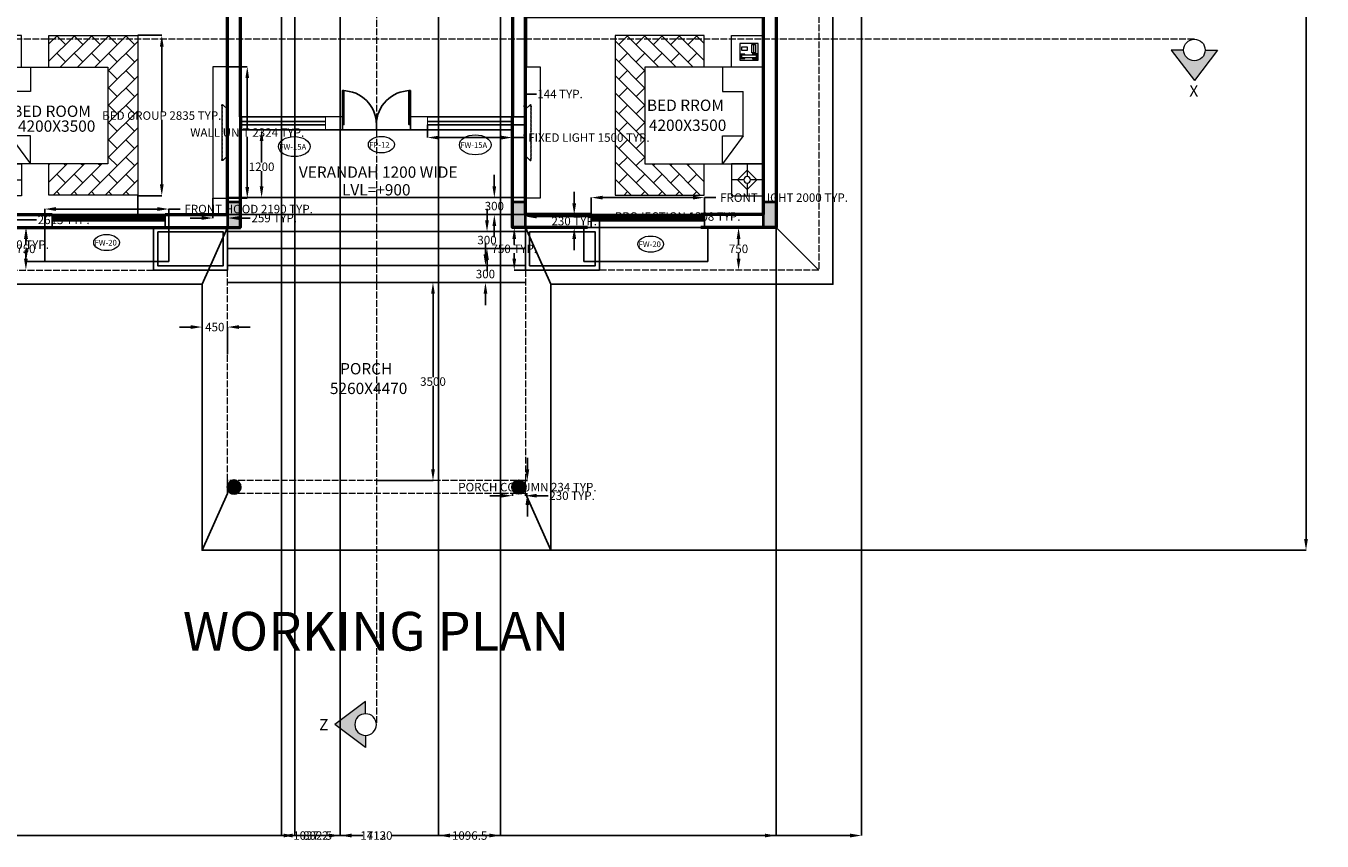
# Model space of a CAD drawing. Units: inches. Extents: x 22626 to 57351, y 2118 to 36234.
# Tile 3 of 10: x 34432 to 57323, y 2118 to 16521. Entities that reach past the tile are written whole.
import ezdxf

# ---------------------------------------------------------------- set-up
doc = ezdxf.new("R2010")
doc.units = ezdxf.units.IN
doc.header["$MEASUREMENT"] = 0
doc.linetypes.add('ACAD_ISO02W100', pattern=[15, 12, -3])
for name, color, linetype, lineweight in [('A-ANNO-DIMS', 130, 'Continuous', 18), ('A-ANNO-IDEN', 130, 'Continuous', 15), ('A-ANNO-SYMB', 130, 'Continuous', 18), ('A-ANNO-TITL', 130, 'Continuous', 35), ('A-AREA-IDEN', 130, 'Continuous', 18), ('A-COLS', 7, 'Continuous', 40), ('A-ROOF', 80, 'Continuous', 25), ('A-ROOF-OVHD', 80, 'ACAD_ISO02W100', 18), ('A-WALL', 80, 'Continuous', 50), ('DOORS', 32, 'Continuous', 25), ('FURNITURE', 30, 'Continuous', 18), ('STAIRS', 82, 'Continuous', 25), ('WINDOWS', 212, 'Continuous', 25)]:
    doc.layers.add(name, color=color, linetype=linetype, lineweight=lineweight)
doc.layers.add('A-SECT', color=2, linetype='ACAD_ISO02W100', lineweight=18, true_color=0xf1eb1f)
doc.styles.get("Standard").update_dxf_attribs({"font": 'arial.ttf'})
doc.dimstyles.get("Standard").update_dxf_attribs({"dimtxt": 150, "dimasz": 200, "dimexe": 0.18, "dimexo": 0.0625, "dimgap": 0.09, "dimtad": 0, "dimtih": 1, "dimtoh": 1, "dimdec": 0, "dimzin": 0, "dimdsep": 46, "dimtxsty": 'Standard', "dimcen": 0.09, "dimadec": 0, "dimazin": 0, "dimtfac": 1, "dimtdec": 0, "dimtofl": 0, "dimtmove": 0, "dimatfit": 3, "dimfxl": 1, "dimtolj": 1, "dimtzin": 0, "dimarcsym": 0})

# ---------------------------------------------------------------- blocks, each defined once
blk = doc.blocks.new('*D1')
at = {"layer": 'A-ANNO-DIMS', "color": 0, "lineweight": -2, "transparency": 16777216}
for p, q in [((40622, 11987), (41621, 11987)), ((41621, 11787), (41621, 10314)), ((41621, 8687), (41621, 10160)), ((40622, 8487), (41621, 8487))]:
    blk.add_line(p, q, dxfattribs=at)
at = {"layer": 'A-ANNO-DIMS', "color": 0, "transparency": 16777216}
for points in [[(41587, 11787), (41654, 11787), (41621, 11987)], [(41587, 8687), (41654, 8687), (41621, 8487)]]:
    blk.add_solid(points, dxfattribs=at)
at = {"layer": 'Defpoints', "color": 0, "transparency": 16777216}
for p in [(40622, 11987), (40622, 8487), (41621, 8487)]:
    blk.add_point(p, dxfattribs=at)
at = {"layer": 'A-ANNO-DIMS', "color": 0, "transparency": 16777216, "insert": (41621, 10237), "char_height": 150, "attachment_point": 5}
blk.add_mtext('\\A1;3500', dxfattribs=at)
blk = doc.blocks.new('*D2')
at = {"layer": 'A-ANNO-DIMS', "color": 0, "lineweight": -2, "transparency": 16777216}
for p, q in [((37342, 11200), (37142, 11200)), ((37542, 10722), (37542, 11200)), ((37992, 10722), (37992, 11200)), ((38192, 11200), (38392, 11200))]:
    blk.add_line(p, q, dxfattribs=at)
at = {"layer": 'A-ANNO-DIMS', "color": 0, "transparency": 16777216}
for points in [[(37342, 11233), (37342, 11167), (37542, 11200)], [(38192, 11233), (38192, 11167), (37992, 11200)]]:
    blk.add_solid(points, dxfattribs=at)
at = {"layer": 'Defpoints', "color": 0, "transparency": 16777216}
for p in [(37542, 11200), (37542, 10722), (37992, 10722)]:
    blk.add_point(p, dxfattribs=at)
at = {"layer": 'A-ANNO-DIMS', "color": 0, "transparency": 16777216, "insert": (37767, 11200), "char_height": 150, "attachment_point": 5}
blk.add_mtext('\\A1;450', dxfattribs=at)
blk = doc.blocks.new('*D3')
at = {"layer": 'A-ANNO-DIMS', "color": 0, "lineweight": -2, "transparency": 16777216}
for p, q in [((42547, 12487), (42547, 12687)), ((43252, 12287), (42547, 12287)), ((43252, 11987), (42547, 11987)), ((42547, 11787), (42547, 11587))]:
    blk.add_line(p, q, dxfattribs=at)
at = {"layer": 'A-ANNO-DIMS', "color": 0, "transparency": 16777216}
for points in [[(42514, 12487), (42581, 12487), (42547, 12287)], [(42514, 11787), (42581, 11787), (42547, 11987)]]:
    blk.add_solid(points, dxfattribs=at)
at = {"layer": 'Defpoints', "color": 0, "transparency": 16777216}
for p in [(42547, 12287), (43252, 12287), (43252, 11987)]:
    blk.add_point(p, dxfattribs=at)
at = {"layer": 'A-ANNO-DIMS', "color": 0, "transparency": 16777216, "insert": (42547, 12137), "char_height": 150, "attachment_point": 5}
blk.add_mtext('\\A1;300', dxfattribs=at)
blk = doc.blocks.new('*D4')
at = {"layer": 'A-ANNO-DIMS', "color": 0, "lineweight": -2, "transparency": 16777216}
for p, q in [((42704, 13687), (42704, 13887)), ((43252, 13487), (42704, 13487)), ((43252, 13187), (42704, 13187)), ((42704, 12987), (42704, 12787))]:
    blk.add_line(p, q, dxfattribs=at)
at = {"layer": 'A-ANNO-DIMS', "color": 0, "transparency": 16777216}
for points in [[(42671, 13687), (42737, 13687), (42704, 13487)], [(42671, 12987), (42737, 12987), (42704, 13187)]]:
    blk.add_solid(points, dxfattribs=at)
at = {"layer": 'Defpoints', "color": 0, "transparency": 16777216}
for p in [(43252, 13487), (42704, 13187), (43252, 13187)]:
    blk.add_point(p, dxfattribs=at)
at = {"layer": 'A-ANNO-DIMS', "color": 0, "transparency": 16777216, "insert": (42704, 13337), "char_height": 150, "attachment_point": 5}
blk.add_mtext('\\A1;300', dxfattribs=at)
blk = doc.blocks.new('*D5')
at = {"layer": 'A-ANNO-DIMS', "color": 0, "lineweight": -2, "transparency": 16777216}
for p, q in [((42575, 13087), (42575, 13287)), ((43252, 12887), (42574, 12887)), ((43252, 12587), (42574, 12587)), ((42575, 12387), (42575, 12187))]:
    blk.add_line(p, q, dxfattribs=at)
at = {"layer": 'A-ANNO-DIMS', "color": 0, "transparency": 16777216}
for points in [[(42541, 13087), (42608, 13087), (42575, 12887)], [(42541, 12387), (42608, 12387), (42575, 12587)]]:
    blk.add_solid(points, dxfattribs=at)
at = {"layer": 'Defpoints', "color": 0, "transparency": 16777216}
for p in [(43252, 12887), (42575, 12587), (43252, 12587)]:
    blk.add_point(p, dxfattribs=at)
at = {"layer": 'A-ANNO-DIMS', "color": 0, "transparency": 16777216, "insert": (42575, 12737), "char_height": 150, "attachment_point": 5}
blk.add_mtext('\\A1;300', dxfattribs=at)
blk = doc.blocks.new('Phone - Desk')
for p, q in [((-4.5, -5), (-4.5, 5)), ((-4.5, 5), (4.5, 5)), ((-4, 4.5), (-4, 2)), ((-4, 2), (-3.25, 2)), ((-3.75, 4.5), (-3.75, 2.25)), ((-1.25, 4.5), (-3.75, 4.5)), ((-3.75, 2.25), (-3.25, 2.25)), ((-3.25, 4), (-3.25, -4)), ((-3.25, 4), (-1.75, 4)), ((-1.75, -4), (-1.75, 4)), ((-1.75, 2.25), (-1.25, 2.25)), ((-1.75, 2), (-1, 2)), ((-1.25, 2.25), (-1.25, 4.5)), ((-1, 2), (-1, 4.5)), ((4, 3.5), (-0.5, 3.5)), ((-0.5, 3.5), (-0.5, 1.5)), ((-0.5, 2.5), (4, 2.5)), ((-0.5, 1.5), (4, 1.5)), ((4, 1.5), (4, 3.5)), ((4.5, 5), (4.5, -5)), ((4.5, -5), (-4.5, -5)), ((-3.75, -2.25), (-3.25, -2.25)), ((-3.75, -4.5), (-3.75, -2.25)), ((-1.25, -4.5), (-3.75, -4.5)), ((-3.25, -4), (-1.75, -4)), ((-1.75, -2.25), (-1.25, -2.25)), ((-1.25, -2.25), (-1.25, -4.5)), ((2.75, -1), (0.75, -1)), ((0.75, -1), (0.75, -4)), ((0.75, -4), (2.75, -4)), ((2.75, -4), (2.75, -1))]:
    blk.add_line(p, q)
blk = doc.blocks.new('BED')
h = blk.add_hatch()
h.set_pattern_fill('AR-B816', color=256, scale=27, angle=45)
h.paths.add_polyline_path([(36405, 26901), (36405, 25191), (35361, 25191), (35361, 24640), (36931, 24640), (36931, 25191), (36931, 27463), (36405, 27463), (35361, 27463), (35361, 26901)])
for p, q in [((35361, 26901), (35361, 27463)), ((35361, 27463), (36405, 27463)), ((36405, 27463), (36931, 27463)), ((36931, 27463), (36931, 25191)), ((35035, 26901), (35035, 26469)), ((34673, 25686), (34673, 26469)), ((35035, 26469), (34673, 26469)), ((35035, 25686), (34673, 25686)), ((34673, 25686), (35035, 25191)), ((35035, 25191), (35035, 25686)), ((34599, 25191), (34599, 24968)), ((35361, 24640), (35361, 25191)), ((36931, 25191), (36931, 24640)), ((34429, 24909), (34599, 25080)), ((34599, 25080), (34769, 24909)), ((34317, 24909), (34540, 24909)), ((34599, 24739), (34429, 24909)), ((34769, 24909), (34599, 24739)), ((34599, 24850), (34599, 24628)), ((34658, 24909), (34880, 24909)), ((36931, 24640), (35361, 24640))]:
    blk.add_line(p, q)
for points in [[(34317, 26901), (34880, 26901), (34880, 27463), (34317, 27463)], [(34317, 26901), (36405, 26901), (36405, 25191), (34317, 25191)], [(34317, 25191), (34880, 25191), (34880, 24628), (34317, 24628)]]:
    blk.add_lwpolyline(points, close=True)
blk.add_circle((34599, 24909), 59)
at = {"xscale": 32.52267765020765, "yscale": 32.52267765020765, "zscale": 32.52267765020765, "rotation": 90}
blk.add_blockref('Phone - Desk', (34567, 27173), dxfattribs=at)
blk = doc.blocks.new('*U7')
for p, q in [((0, 0), (0, -6)), ((40, 0), (40, -6))]:
    blk.add_line(p, q)
blk.add_lwpolyline([(0, 0), (0, 40), (1.75, 40), (1.75, 0)], close=True)
blk.add_arc((0, 0), 40, 0, 90)
blk = doc.blocks.new('*D16')
at = {"layer": 'A-ANNO-DIMS', "color": 0, "lineweight": -2, "transparency": 16777216}
for p, q in [((47017, 12957), (47018, 12957)), ((47017, 12757), (47017, 12659)), ((47017, 12407), (47017, 12505)), ((47017, 12207), (47018, 12207))]:
    blk.add_line(p, q, dxfattribs=at)
at = {"layer": 'A-ANNO-DIMS', "color": 0, "transparency": 16777216}
for points in [[(46984, 12757), (47051, 12757), (47017, 12957)], [(46984, 12407), (47051, 12407), (47017, 12207)]]:
    blk.add_solid(points, dxfattribs=at)
at = {"layer": 'Defpoints', "color": 0, "transparency": 16777216}
for p in [(47017, 12957), (47017, 12207), (47017, 12207)]:
    blk.add_point(p, dxfattribs=at)
at = {"layer": 'A-ANNO-DIMS', "color": 0, "transparency": 16777216, "insert": (47017, 12582), "char_height": 150, "attachment_point": 5}
blk.add_mtext('\\A1;750', dxfattribs=at)
blk = doc.blocks.new('*D17')
at = {"layer": 'A-ANNO-DIMS', "color": 0, "lineweight": -2, "transparency": 16777216}
for p, q in [((38594, 14687), (38594, 14687)), ((38594, 14487), (38594, 14108)), ((38594, 13687), (38594, 13955)), ((38594, 13487), (38594, 13487))]:
    blk.add_line(p, q, dxfattribs=at)
at = {"layer": 'A-ANNO-DIMS', "color": 0, "transparency": 16777216}
for points in [[(38561, 14487), (38627, 14487), (38594, 14687)], [(38561, 13687), (38627, 13687), (38594, 13487)]]:
    blk.add_solid(points, dxfattribs=at)
at = {"layer": 'Defpoints', "color": 0, "transparency": 16777216}
for p in [(38594, 14687), (38594, 14687), (38594, 13487)]:
    blk.add_point(p, dxfattribs=at)
at = {"layer": 'A-ANNO-DIMS', "color": 0, "transparency": 16777216, "insert": (38594, 14032), "char_height": 150, "attachment_point": 5}
blk.add_mtext('\\A1;1200', dxfattribs=at)
blk = doc.blocks.new('*D19')
at = {"layer": 'A-ANNO-DIMS', "color": 0, "lineweight": -2, "transparency": 16777216}
for p, q in [((34431, 12957), (34431, 12957)), ((34431, 12757), (34431, 12659)), ((34431, 12407), (34431, 12505)), ((34431, 12207), (34431, 12207))]:
    blk.add_line(p, q, dxfattribs=at)
at = {"layer": 'A-ANNO-DIMS', "color": 0, "transparency": 16777216}
for points in [[(34398, 12757), (34464, 12757), (34431, 12957)], [(34398, 12407), (34464, 12407), (34431, 12207)]]:
    blk.add_solid(points, dxfattribs=at)
at = {"layer": 'Defpoints', "color": 0, "transparency": 16777216}
for p in [(34431, 12957), (34431, 12207), (34431, 12207)]:
    blk.add_point(p, dxfattribs=at)
at = {"layer": 'A-ANNO-DIMS', "color": 0, "transparency": 16777216, "insert": (34431, 12582), "char_height": 150, "attachment_point": 5}
blk.add_mtext('\\A1;750', dxfattribs=at)
blk = doc.blocks.new('BEDROOM-WALL-UNIT-SMALL')
for p, q in [((259, 1576), (175, 1654)), ((259, 1576), (259, 748)), ((259, 748), (175, 670))]:
    blk.add_line(p, q)
blk.add_lwpolyline([(259, 2324), (0, 2324), (0, 0), (259, 0)], close=True)
for centre in [(168, 1645), (168, 679)]:
    blk.add_circle(centre, 11.7)
for centre, radius, start, end in [((170, 1620), 14.3, 99.4783, 260.5217), ((168, 1594), 11.7, 90, 270), ((168, 1570), 11.7, 90, 270), ((168, 1547), 11.7, 90, 270), ((168, 1523), 11.7, 90, 270), ((168, 1500), 11.7, 90, 270), ((168, 1476), 11.7, 90, 270), ((168, 1453), 11.7, 90, 270), ((168, 1430), 11.7, 90, 270), ((168, 1406), 11.7, 90, 270), ((168, 1383), 11.7, 90, 270), ((168, 1359), 11.7, 90, 270), ((168, 1336), 11.7, 90, 270), ((168, 1312), 11.7, 90, 270), ((168, 1289), 11.7, 90, 270), ((168, 1265), 11.7, 90, 270), ((168, 1242), 11.7, 90, 270), ((168, 1218), 11.7, 90, 270), ((168, 1195), 11.7, 90, 270), ((168, 1172), 11.7, 90, 270), ((168, 1148), 11.7, 90, 270), ((168, 1125), 11.7, 90, 270), ((168, 1101), 11.7, 90, 270), ((168, 1078), 11.7, 90, 270), ((168, 1054), 11.7, 90, 270), ((168, 1031), 11.7, 90, 270), ((168, 1007), 11.7, 90, 270), ((168, 984), 11.7, 90, 270), ((168, 960), 11.7, 90, 270), ((168, 937), 11.7, 90, 270), ((168, 914), 11.7, 90, 270), ((168, 890), 11.7, 90, 270), ((168, 867), 11.7, 90, 270), ((168, 843), 11.7, 90, 270), ((168, 820), 11.7, 90, 270), ((168, 796), 11.7, 90, 270), ((168, 773), 11.7, 90, 270), ((168, 749), 11.7, 90, 270), ((168, 726), 11.7, 90, 270), ((168, 702), 11.7, 90, 270)]:
    blk.add_arc(centre, radius, start, end)
blk = doc.blocks.new('WIN-FIXED-2000-FRONT')
for p, q in [((0, 207), (2000, 207)), ((0, 177), (2000, 177)), ((0, 147), (2000, 147)), ((0, 117), (2000, 117))]:
    blk.add_line(p, q)
blk.add_lwpolyline([(0, 230), (2000, 230), (2000, 0), (0, 0), (0, 230)])
blk = doc.blocks.new('COL-RECTANGULAR')
h = blk.add_hatch(color=256)
h.dxf.hatch_style = 1
h.paths.add_polyline_path([(0, 0), (450, 0), (450, 230), (0, 230)])
blk.add_lwpolyline([(0, 0), (0, 230), (450, 230), (450, 0)], close=True)
blk = doc.blocks.new('COL-ROUND')
h = blk.add_hatch(color=256)
h.dxf.hatch_style = 1
h.paths.add_polyline_path([(0, 115, 0.970679), (230, 108), (230, 122, 0.970679)])
blk.add_circle((115, 115), 115)
blk = doc.blocks.new('SECTION-HEAD')
h = blk.add_hatch(color=256)
h.dxf.hatch_style = 1
h.paths.add_polyline_path([(815, 541), (599, 541, -1), (216, 541), (0, 541), (407, 0)])
for p, q in [((216, 541), (0, 541)), ((0, 541), (407, 0)), ((815, 541), (407, 0)), ((599, 541), (815, 541))]:
    blk.add_line(p, q)
blk.add_circle((407, 541), 191)
blk = doc.blocks.new('WINDOW-HOOD-FRONT')
for p, q in [((0, 0), (0, 600)), ((2190, 600), (2190, 0)), ((2190, 0), (0, 0))]:
    blk.add_line(p, q)
blk = doc.blocks.new('FRONT-PROJECTION')
for points in [[(0, 750), (1308, 750), (1308, 0), (0, 0)], [(75, 675), (1233, 675), (1233, 75), (75, 75)]]:
    blk.add_lwpolyline(points, close=True)
blk = doc.blocks.new('WIN-FIXED-1500')
for p, q in [((1500, 144), (0, 144)), ((0, 58), (1500, 58)), ((0, 0), (1500, 0))]:
    blk.add_line(p, q)
blk = doc.blocks.new('*D58')
at = {"layer": 'A-ANNO-DIMS', "color": 0, "lineweight": -2, "transparency": 16777216}
for p, q in [((43288, 8689), (43288, 8889)), ((43253, 8489), (43288, 8489)), ((43253, 8255), (43288, 8255)), ((43288, 8055), (43288, 7855))]:
    blk.add_line(p, q, dxfattribs=at)
at = {"layer": 'A-ANNO-DIMS', "color": 0, "transparency": 16777216}
for points in [[(43254, 8689), (43321, 8689), (43288, 8489)], [(43254, 8055), (43321, 8055), (43288, 8255)]]:
    blk.add_solid(points, dxfattribs=at)
at = {"layer": 'Defpoints', "color": 0, "transparency": 16777216}
for p in [(43253, 8489), (43288, 8489), (43253, 8255)]:
    blk.add_point(p, dxfattribs=at)
at = {"layer": 'A-ANNO-DIMS', "color": 0, "transparency": 16777216, "insert": (43288, 8372), "char_height": 150, "attachment_point": 5}
blk.add_mtext('\\A1;PORCH COLUMN 234 TYP.', dxfattribs=at)
blk = doc.blocks.new('*D59')
at = {"layer": 'A-ANNO-DIMS', "color": 0, "lineweight": -2, "transparency": 16777216}
for p, q in [((43023, 8255), (43023, 8220)), ((43253, 8255), (43253, 8220)), ((42823, 8220), (42623, 8220)), ((43453, 8220), (43653, 8220))]:
    blk.add_line(p, q, dxfattribs=at)
at = {"layer": 'A-ANNO-DIMS', "color": 0, "transparency": 16777216}
for points in [[(42823, 8253), (42823, 8187), (43023, 8220)], [(43453, 8253), (43453, 8187), (43253, 8220)]]:
    blk.add_solid(points, dxfattribs=at)
at = {"layer": 'Defpoints', "color": 0, "transparency": 16777216}
for p in [(43023, 8255), (43253, 8255), (43253, 8220)]:
    blk.add_point(p, dxfattribs=at)
at = {"layer": 'A-ANNO-DIMS', "color": 0, "transparency": 16777216, "insert": (44077, 8220), "char_height": 150, "attachment_point": 5}
blk.add_mtext('\\A1;230 TYP.', dxfattribs=at)
blk = doc.blocks.new('*D60')
at = {"layer": 'A-ANNO-DIMS', "color": 0, "lineweight": -2, "transparency": 16777216}
for p, q in [((36406, 16355), (36831, 16355)), ((36831, 16155), (36831, 15015)), ((36831, 13719), (36831, 14859)), ((36406, 13519), (36831, 13519))]:
    blk.add_line(p, q, dxfattribs=at)
at = {"layer": 'A-ANNO-DIMS', "color": 0, "transparency": 16777216}
for points in [[(36798, 16155), (36864, 16155), (36831, 16355)], [(36798, 13719), (36864, 13719), (36831, 13519)]]:
    blk.add_solid(points, dxfattribs=at)
at = {"layer": 'Defpoints', "color": 0, "transparency": 16777216}
for p in [(36406, 16355), (36831, 16355), (36406, 13519)]:
    blk.add_point(p, dxfattribs=at)
at = {"layer": 'A-ANNO-DIMS', "color": 0, "transparency": 16777216, "insert": (36831, 14937), "char_height": 150, "attachment_point": 5}
blk.add_mtext('\\A1;BED GROUP 2835 TYP.', dxfattribs=at)
blk = doc.blocks.new('*D61')
at = {"layer": 'A-ANNO-DIMS', "color": 0, "lineweight": -2, "transparency": 16777216}
for p, q in [((33792, 13519), (33792, 13094)), ((36406, 13519), (36406, 13094)), ((33992, 13094), (34616, 13094)), ((36206, 13094), (35582, 13094))]:
    blk.add_line(p, q, dxfattribs=at)
at = {"layer": 'A-ANNO-DIMS', "color": 0, "transparency": 16777216}
for points in [[(33992, 13127), (33992, 13061), (33792, 13094)], [(36206, 13127), (36206, 13061), (36406, 13094)]]:
    blk.add_solid(points, dxfattribs=at)
at = {"layer": 'Defpoints', "color": 0, "transparency": 16777216}
for p in [(33792, 13519), (36406, 13519), (36406, 13094)]:
    blk.add_point(p, dxfattribs=at)
at = {"layer": 'A-ANNO-DIMS', "color": 0, "transparency": 16777216, "insert": (35099, 13094), "char_height": 150, "attachment_point": 5}
blk.add_mtext('\\A1;2613 TYP.', dxfattribs=at)
blk = doc.blocks.new('*D80')
at = {"layer": 'A-ANNO-DIMS', "color": 0, "lineweight": -2, "transparency": 16777216}
for p, q in [((37992, 15799), (38341, 15799)), ((38341, 15599), (38341, 14714)), ((38341, 13675), (38341, 14560)), ((37992, 13475), (38341, 13475))]:
    blk.add_line(p, q, dxfattribs=at)
at = {"layer": 'A-ANNO-DIMS', "color": 0, "transparency": 16777216}
for points in [[(38308, 15599), (38374, 15599), (38341, 15799)], [(38308, 13675), (38374, 13675), (38341, 13475)]]:
    blk.add_solid(points, dxfattribs=at)
at = {"layer": 'Defpoints', "color": 0, "transparency": 16777216}
for p in [(37992, 15799), (38341, 15799), (37992, 13475)]:
    blk.add_point(p, dxfattribs=at)
at = {"layer": 'A-ANNO-DIMS', "color": 0, "transparency": 16777216, "insert": (38341, 14637), "char_height": 150, "attachment_point": 5}
blk.add_mtext('\\A1;WALL UNIT 2324 TYP.', dxfattribs=at)
blk = doc.blocks.new('*D81')
at = {"layer": 'A-ANNO-DIMS', "color": 0, "lineweight": -2, "transparency": 16777216}
for p, q in [((37734, 13475), (37734, 13126)), ((37992, 13475), (37992, 13126)), ((37534, 13126), (37334, 13126)), ((38192, 13126), (38392, 13126))]:
    blk.add_line(p, q, dxfattribs=at)
at = {"layer": 'A-ANNO-DIMS', "color": 0, "transparency": 16777216}
for points in [[(37534, 13159), (37534, 13093), (37734, 13126)], [(38192, 13159), (38192, 13093), (37992, 13126)]]:
    blk.add_solid(points, dxfattribs=at)
at = {"layer": 'Defpoints', "color": 0, "transparency": 16777216}
for p in [(37734, 13475), (37992, 13475), (37992, 13126)]:
    blk.add_point(p, dxfattribs=at)
at = {"layer": 'A-ANNO-DIMS', "color": 0, "transparency": 16777216, "insert": (38817, 13126), "char_height": 150, "attachment_point": 5}
blk.add_mtext('\\A1;259 TYP.', dxfattribs=at)
blk = doc.blocks.new('*D84')
at = {"layer": 'A-ANNO-DIMS', "color": 0, "lineweight": -2, "transparency": 16777216}
for p, q in [((44415, 13187), (44415, 13487)), ((44615, 13487), (46215, 13487)), ((46415, 13187), (46415, 13487)), ((46415, 13487), (46615, 13487))]:
    blk.add_line(p, q, dxfattribs=at)
at = {"layer": 'A-ANNO-DIMS', "color": 0, "transparency": 16777216}
for points in [[(44615, 13520), (44615, 13454), (44415, 13487)], [(46215, 13520), (46215, 13454), (46415, 13487)]]:
    blk.add_solid(points, dxfattribs=at)
at = {"layer": 'Defpoints', "color": 0, "transparency": 16777216}
for p in [(46415, 13487), (44415, 13187), (46415, 13187)]:
    blk.add_point(p, dxfattribs=at)
at = {"layer": 'A-ANNO-DIMS', "color": 0, "transparency": 16777216, "insert": (47821, 13487), "char_height": 150, "attachment_point": 5}
blk.add_mtext('\\A1;FRONT LIGHT 2000 TYP.', dxfattribs=at)
blk = doc.blocks.new('*D85')
at = {"layer": 'A-ANNO-DIMS', "color": 0, "lineweight": -2, "transparency": 16777216}
for p, q in [((44115, 13387), (44115, 13587)), ((44415, 13187), (44115, 13187)), ((44415, 12957), (44115, 12957)), ((44115, 12757), (44115, 12557))]:
    blk.add_line(p, q, dxfattribs=at)
at = {"layer": 'A-ANNO-DIMS', "color": 0, "transparency": 16777216}
for points in [[(44082, 13387), (44149, 13387), (44115, 13187)], [(44082, 12757), (44149, 12757), (44115, 12957)]]:
    blk.add_solid(points, dxfattribs=at)
at = {"layer": 'Defpoints', "color": 0, "transparency": 16777216}
for p in [(44115, 13187), (44415, 13187), (44415, 12957)]:
    blk.add_point(p, dxfattribs=at)
at = {"layer": 'A-ANNO-DIMS', "color": 0, "transparency": 16777216, "insert": (44115, 13072), "char_height": 150, "attachment_point": 5}
blk.add_mtext('\\A1;230 TYP.', dxfattribs=at)
blk = doc.blocks.new('*D88')
at = {"layer": 'A-ANNO-DIMS', "color": 0, "lineweight": -2, "transparency": 16777216}
for p, q in [((34763, 12957), (34763, 13286)), ((34963, 13285), (36754, 13285)), ((36954, 12957), (36954, 13286)), ((36954, 13285), (37154, 13285))]:
    blk.add_line(p, q, dxfattribs=at)
at = {"layer": 'A-ANNO-DIMS', "color": 0, "transparency": 16777216}
for points in [[(34963, 13319), (34963, 13252), (34763, 13285)], [(36754, 13319), (36754, 13252), (36954, 13285)]]:
    blk.add_solid(points, dxfattribs=at)
at = {"layer": 'Defpoints', "color": 0, "transparency": 16777216}
for p in [(36954, 13285), (34763, 12957), (36954, 12957)]:
    blk.add_point(p, dxfattribs=at)
at = {"layer": 'A-ANNO-DIMS', "color": 0, "transparency": 16777216, "insert": (38365, 13285), "char_height": 150, "attachment_point": 5}
blk.add_mtext('\\A1;FRONT HOOD 2190 TYP.', dxfattribs=at)
blk = doc.blocks.new('*D89')
at = {"layer": 'A-ANNO-DIMS', "color": 0, "lineweight": -2, "transparency": 16777216}
for p, q in [((34763, 12957), (34435, 12957)), ((34435, 12757), (34435, 12734)), ((34435, 12557), (34435, 12580)), ((34763, 12357), (34435, 12357))]:
    blk.add_line(p, q, dxfattribs=at)
at = {"layer": 'A-ANNO-DIMS', "color": 0, "transparency": 16777216}
for points in [[(34401, 12757), (34468, 12757), (34435, 12957)], [(34401, 12557), (34468, 12557), (34435, 12357)]]:
    blk.add_solid(points, dxfattribs=at)
at = {"layer": 'Defpoints', "color": 0, "transparency": 16777216}
for p in [(34435, 12957), (34763, 12957), (34763, 12357)]:
    blk.add_point(p, dxfattribs=at)
at = {"layer": 'A-ANNO-DIMS', "color": 0, "transparency": 16777216, "insert": (34435, 12657), "char_height": 150, "attachment_point": 5}
blk.add_mtext('\\A1;600 TYP.', dxfattribs=at)
blk = doc.blocks.new('*D90')
at = {"layer": 'A-ANNO-DIMS', "color": 0, "lineweight": -2, "transparency": 16777216}
for p, q in [((43252, 12957), (43252, 13153)), ((43452, 13153), (44361, 13153)), ((44561, 12957), (44561, 13153)), ((44561, 13153), (44761, 13153))]:
    blk.add_line(p, q, dxfattribs=at)
at = {"layer": 'A-ANNO-DIMS', "color": 0, "transparency": 16777216}
for points in [[(43452, 13186), (43452, 13120), (43252, 13153)], [(44361, 13186), (44361, 13120), (44561, 13153)]]:
    blk.add_solid(points, dxfattribs=at)
at = {"layer": 'Defpoints', "color": 0, "transparency": 16777216}
for p in [(44561, 13153), (43252, 12957), (44561, 12957)]:
    blk.add_point(p, dxfattribs=at)
at = {"layer": 'A-ANNO-DIMS', "color": 0, "transparency": 16777216, "insert": (45943, 13153), "char_height": 150, "attachment_point": 5}
blk.add_mtext('\\A1;PROJECTION 1308 TYP.', dxfattribs=at)
blk = doc.blocks.new('*D91')
at = {"layer": 'A-ANNO-DIMS', "color": 0, "lineweight": -2, "transparency": 16777216}
for p, q in [((43252, 12957), (43056, 12957)), ((43056, 12757), (43056, 12659)), ((43056, 12407), (43056, 12505)), ((43252, 12207), (43056, 12207))]:
    blk.add_line(p, q, dxfattribs=at)
at = {"layer": 'A-ANNO-DIMS', "color": 0, "transparency": 16777216}
for points in [[(43023, 12757), (43089, 12757), (43056, 12957)], [(43023, 12407), (43089, 12407), (43056, 12207)]]:
    blk.add_solid(points, dxfattribs=at)
at = {"layer": 'Defpoints', "color": 0, "transparency": 16777216}
for p in [(43056, 12957), (43252, 12957), (43252, 12207)]:
    blk.add_point(p, dxfattribs=at)
at = {"layer": 'A-ANNO-DIMS', "color": 0, "transparency": 16777216, "insert": (43056, 12582), "char_height": 150, "attachment_point": 5}
blk.add_mtext('\\A1;750 TYP.', dxfattribs=at)
blk = doc.blocks.new('*D96')
at = {"layer": 'A-ANNO-DIMS', "color": 0, "lineweight": -2, "transparency": 16777216}
for p, q in [((41522, 14773), (41522, 14547)), ((43022, 14773), (43022, 14547)), ((41722, 14548), (42822, 14548)), ((43022, 14548), (43222, 14548))]:
    blk.add_line(p, q, dxfattribs=at)
at = {"layer": 'A-ANNO-DIMS', "color": 0, "transparency": 16777216}
for points in [[(41722, 14581), (41722, 14514), (41522, 14548)], [(42822, 14581), (42822, 14514), (43022, 14548)]]:
    blk.add_solid(points, dxfattribs=at)
at = {"layer": 'Defpoints', "color": 0, "transparency": 16777216}
for p in [(41522, 14773), (43022, 14773), (43022, 14548)]:
    blk.add_point(p, dxfattribs=at)
at = {"layer": 'A-ANNO-DIMS', "color": 0, "transparency": 16777216, "insert": (44375, 14548), "char_height": 150, "attachment_point": 5}
blk.add_mtext('\\A1;FIXED LIGHT 1500 TYP.', dxfattribs=at)
blk = doc.blocks.new('*D97')
at = {"layer": 'A-ANNO-DIMS', "color": 0, "lineweight": -2, "transparency": 16777216}
for p, q in [((43247, 15117), (43247, 15317)), ((43247, 15317), (43447, 15317)), ((43022, 14917), (43248, 14917)), ((43022, 14773), (43248, 14773)), ((43247, 14573), (43247, 14373))]:
    blk.add_line(p, q, dxfattribs=at)
at = {"layer": 'A-ANNO-DIMS', "color": 0, "transparency": 16777216}
for points in [[(43214, 15117), (43281, 15117), (43247, 14917)], [(43214, 14573), (43281, 14573), (43247, 14773)]]:
    blk.add_solid(points, dxfattribs=at)
at = {"layer": 'Defpoints', "color": 0, "transparency": 16777216}
for p in [(43022, 14917), (43247, 14917), (43022, 14773)]:
    blk.add_point(p, dxfattribs=at)
at = {"layer": 'A-ANNO-DIMS', "color": 0, "transparency": 16777216, "insert": (43864, 15317), "char_height": 150, "attachment_point": 5}
blk.add_mtext('\\A1;144 TYP.', dxfattribs=at)
blk = doc.blocks.new('*D99')
at = {"layer": 'A-ANNO-DIMS', "color": 0, "lineweight": -2, "transparency": 16777216}
for p, q in [((41185, 30457), (57039, 30457)), ((57039, 30257), (57039, 18934)), ((57039, 7457), (57039, 18780)), ((43702, 7257), (57039, 7257))]:
    blk.add_line(p, q, dxfattribs=at)
at = {"layer": 'A-ANNO-DIMS', "color": 0, "transparency": 16777216}
for points in [[(57005, 30257), (57072, 30257), (57039, 30457)], [(57005, 7457), (57072, 7457), (57039, 7257)]]:
    blk.add_solid(points, dxfattribs=at)
at = {"layer": 'Defpoints', "color": 0, "transparency": 16777216}
for p in [(41185, 30457), (57039, 30457), (43702, 7257)]:
    blk.add_point(p, dxfattribs=at)
at = {"layer": 'A-ANNO-DIMS', "color": 0, "transparency": 16777216, "insert": (57039, 18857), "char_height": 150, "attachment_point": 5}
blk.add_mtext('\\A1;23200', dxfattribs=at)
blk = doc.blocks.new('*D100')
at = {"layer": 'A-ANNO-DIMS', "color": 0, "lineweight": -2, "transparency": 16777216}
for p, q in [((32057, 23297), (32057, 2216)), ((49187, 23297), (49187, 2216)), ((32257, 2216), (40347, 2216)), ((48987, 2216), (40897, 2216))]:
    blk.add_line(p, q, dxfattribs=at)
at = {"layer": 'A-ANNO-DIMS', "color": 0, "transparency": 16777216}
for points in [[(32257, 2250), (32257, 2183), (32057, 2216)], [(48987, 2250), (48987, 2183), (49187, 2216)]]:
    blk.add_solid(points, dxfattribs=at)
at = {"layer": 'Defpoints', "color": 0, "transparency": 16777216}
for p in [(32057, 23297), (49187, 23297), (49187, 2216)]:
    blk.add_point(p, dxfattribs=at)
at = {"layer": 'A-ANNO-DIMS', "color": 0, "transparency": 16777216, "insert": (40622, 2216), "char_height": 150, "attachment_point": 5}
blk.add_mtext('\\A1;17130', dxfattribs=at)
blk = doc.blocks.new('*D102')
at = {"layer": 'A-ANNO-DIMS', "color": 0, "lineweight": -2, "transparency": 16777216}
for p, q in [((41719, 19741), (41719, 2216)), ((42816, 19741), (42816, 2216)), ((41919, 2216), (41963, 2216)), ((42616, 2216), (42572, 2216))]:
    blk.add_line(p, q, dxfattribs=at)
at = {"layer": 'A-ANNO-DIMS', "color": 0, "transparency": 16777216}
for points in [[(41919, 2250), (41919, 2183), (41719, 2216)], [(42616, 2250), (42616, 2183), (42816, 2216)]]:
    blk.add_solid(points, dxfattribs=at)
at = {"layer": 'Defpoints', "color": 0, "transparency": 16777216}
for p in [(41719, 19741), (42816, 19741), (42816, 2216)]:
    blk.add_point(p, dxfattribs=at)
at = {"layer": 'A-ANNO-DIMS', "color": 0, "transparency": 16777216, "insert": (42268, 2216), "char_height": 150, "attachment_point": 5}
blk.add_mtext('\\A1;1096.5', dxfattribs=at)
blk = doc.blocks.new('*D104')
at = {"layer": 'A-ANNO-DIMS', "color": 0, "lineweight": -2, "transparency": 16777216}
for p, q in [((39181, 20280), (39181, 2216)), ((39983, 20280), (39983, 2216)), ((38981, 2216), (38781, 2216)), ((40183, 2216), (40383, 2216))]:
    blk.add_line(p, q, dxfattribs=at)
at = {"layer": 'A-ANNO-DIMS', "color": 0, "transparency": 16777216}
for points in [[(38981, 2250), (38981, 2183), (39181, 2216)], [(40183, 2250), (40183, 2183), (39983, 2216)]]:
    blk.add_solid(points, dxfattribs=at)
at = {"layer": 'Defpoints', "color": 0, "transparency": 16777216}
for p in [(39181, 20280), (39983, 20280), (39983, 2216)]:
    blk.add_point(p, dxfattribs=at)
at = {"layer": 'A-ANNO-DIMS', "color": 0, "transparency": 16777216, "insert": (39582, 2216), "char_height": 150, "attachment_point": 5}
blk.add_mtext('\\A1;802.5', dxfattribs=at)
blk = doc.blocks.new('*D110')
at = {"layer": 'A-ANNO-DIMS', "color": 0, "lineweight": -2, "transparency": 16777216}
for p, q in [((38945, 27403), (38945, 2216)), ((39982, 27403), (39982, 2216)), ((39145, 2216), (39160, 2216)), ((39782, 2216), (39767, 2216))]:
    blk.add_line(p, q, dxfattribs=at)
at = {"layer": 'A-ANNO-DIMS', "color": 0, "transparency": 16777216}
for points in [[(39145, 2250), (39145, 2183), (38945, 2216)], [(39782, 2250), (39782, 2183), (39982, 2216)]]:
    blk.add_solid(points, dxfattribs=at)
at = {"layer": 'Defpoints', "color": 0, "transparency": 16777216}
for p in [(38945, 27403), (39982, 27403), (39982, 2216)]:
    blk.add_point(p, dxfattribs=at)
at = {"layer": 'A-ANNO-DIMS', "color": 0, "transparency": 16777216, "insert": (39464, 2216), "char_height": 150, "attachment_point": 5}
blk.add_mtext('\\A1;1037.2', dxfattribs=at)
blk = doc.blocks.new('*D113')
at = {"layer": 'A-ANNO-DIMS', "color": 0, "lineweight": -2, "transparency": 16777216}
for p, q in [((33562, 12957), (33562, 2216)), ((47682, 12957), (47682, 2216)), ((33762, 2216), (40347, 2216)), ((47482, 2216), (40897, 2216))]:
    blk.add_line(p, q, dxfattribs=at)
at = {"layer": 'A-ANNO-DIMS', "color": 0, "transparency": 16777216}
for points in [[(33762, 2250), (33762, 2183), (33562, 2216)], [(47482, 2250), (47482, 2183), (47682, 2216)]]:
    blk.add_solid(points, dxfattribs=at)
at = {"layer": 'Defpoints', "color": 0, "transparency": 16777216}
for p in [(33562, 12957), (47682, 12957), (47682, 2216)]:
    blk.add_point(p, dxfattribs=at)
at = {"layer": 'A-ANNO-DIMS', "color": 0, "transparency": 16777216, "insert": (40622, 2216), "char_height": 150, "attachment_point": 5}
blk.add_mtext('\\A1;14120', dxfattribs=at)

msp = doc.modelspace()

# ---------------------------------------------------------------- linework, layer by layer
at = {"layer": 'A-ANNO-IDEN'}
for centre, major_axis in [((39170.63, 14388.14), (279.17, 0)), ((40709.55, 14422.81), (230.24, 0)), ((42366.56, 14419.65), (279.17, 0)), ((35855.61, 12693.22), (226.15, 0)), ((45464.46, 12664.97), (226.15, 0))]:
    msp.add_ellipse(centre, major_axis=major_axis, ratio=0.63425497, start_param=-1.57079633, end_param=4.71238898, dxfattribs=at)
at = {"layer": 'A-ROOF'}
for p, q in [((37542.43, 11956.86), (37992.43, 12956.86)), ((43252.43, 12956.86), (43702.43, 11956.86)), ((48432.43, 12206.86), (47682.43, 12956.86)), ((37992.43, 8256.86), (37542.43, 7256.86)), ((43252.43, 8256.86), (43702.43, 7256.86))]:
    msp.add_line(p, q, dxfattribs=at)
for points in [[(43702.43, 11956.86), (43702.43, 7256.86), (37542.43, 7256.86), (37542.43, 11956.86), (32562.43, 11956.86), (32562.43, 22296.86), (30057.43, 22296.86), (30057.43, 24356.86), (30057.43, 30256.86), (39684.53, 30256.86)], [(41184.53, 30256.86), (50187.43, 30256.86), (50187.43, 25126.86), (50187.43, 22296.86), (48682.43, 22296.86), (48682.43, 11956.86), (43702.43, 11956.86)]]:
    msp.add_lwpolyline(points, dxfattribs=at)
at = {"layer": 'A-ROOF-OVHD', "ltscale": 10}
for p, q in [((48432.43, 18796.86), (48432.43, 12206.86)), ((32812.43, 12206.86), (37992.43, 12206.86)), ((32812.43, 12206.86), (37992.43, 12206.86)), ((48432.43, 12206.86), (43252.43, 12206.86)), ((37992.43, 8256.86), (37992.43, 8486.86)), ((43252.43, 8256.86), (43252.43, 8486.86)), ((43252.43, 8256.86), (37992.43, 8256.86))]:
    msp.add_line(p, q, dxfattribs=at)
msp.add_lwpolyline([(43252.43, 12956.86), (43252.43, 8486.86), (37992.43, 8486.86), (37992.43, 12956.86)], dxfattribs=at)
at = {"layer": 'A-SECT', "ltscale": 10}
for p, q in [((40622.43, 34176.08), (40622.43, 4176.35)), ((55067.61, 16286.11), (24870.06, 16286.11))]:
    msp.add_line(p, q, dxfattribs=at)
at = {"layer": 'A-WALL'}
for p, q in [((43252.43, 18796.86), (43252.43, 15798.95)), ((38222.43, 14916.86), (38222.43, 18566.86)), ((43022.43, 18566.86), (43022.43, 14916.86)), ((37992.43, 13186.86), (37992.43, 16686.86)), ((38222.43, 14916.86), (38222.43, 14686.86)), ((38222.43, 12956.86), (38222.43, 14686.86)), ((33792.43, 13186.86), (34892.43, 13186.86)), ((36892.43, 13186.86), (37987.43, 13186.86)), ((33562.43, 12956.86), (38222.43, 12956.86))]:
    msp.add_line(p, q, dxfattribs=at)
for points in [[(37992.43, 14686.86), (37992.43, 18796.86)], [(47682.43, 16916.86), (47682.43, 12956.86), (46352.43, 12956.86)], [(44415.49, 13186.86), (43252.43, 13186.86), (43252.43, 16686.86), (47452.43, 16686.86), (47452.43, 13186.86), (46352.43, 13186.86)], [(44352.43, 12956.86), (43022.43, 12956.86), (43022.43, 14916.86)]]:
    msp.add_lwpolyline(points, dxfattribs=at)
at = {"layer": 'A-WALL', "const_width": 20}
for points in [[(40022.43, 14916.72), (39722.43, 14916.72), (39722.43, 14686.86), (40022.43, 14686.86)], [(41222.43, 14916.72), (41522.43, 14916.72), (41522.43, 14686.86), (41222.43, 14686.86)]]:
    msp.add_lwpolyline(points, close=True, dxfattribs=at)
at = {"layer": 'STAIRS'}
for p, q in [((43252.43, 13486.86), (37992.43, 13486.86)), ((43252.43, 13186.86), (37992.43, 13186.86)), ((43252.43, 12886.86), (37992.43, 12886.86)), ((43252.43, 12586.86), (37992.43, 12586.86)), ((43252.43, 12286.86), (37992.43, 12286.86)), ((43252.43, 11986.86), (37992.43, 11986.86))]:
    msp.add_line(p, q, dxfattribs=at)
at = {"layer": 'WINDOWS'}
msp.add_line((43022.43, 14686.86), (38222.43, 14686.86), dxfattribs=at)

# ---------------------------------------------------------------- block references
at = {"layer": 'A-ANNO-SYMB'}
msp.add_blockref('SECTION-HEAD', (54660.13, 15553.84), dxfattribs=at)
at = {"layer": 'A-ANNO-SYMB', "extrusion": (0, 0, -1), "zscale": -1, "rotation": 90}
msp.add_blockref('SECTION-HEAD', (-39890.15, 3768.86), dxfattribs=at)
at = {"layer": 'A-COLS', "extrusion": (0, 0, -1), "zscale": -1, "rotation": 90}
for p in [(-37992.43, 12956.86), (-43022.43, 12956.86), (-47452.43, 12956.86)]:
    msp.add_blockref('COL-RECTANGULAR', p, dxfattribs=at)
at = {"layer": 'A-COLS', "extrusion": (0, 0, -1), "zscale": -1}
msp.add_blockref('COL-ROUND', (-38222.23, 8256.86), dxfattribs=at)
at = {"layer": 'A-COLS'}
msp.add_blockref('COL-ROUND', (43022.63, 8256.86), dxfattribs=at)
at = {"layer": 'A-ROOF'}
for name, p in [('WINDOW-HOOD-FRONT', (34763.36, 12356.86)), ('FRONT-PROJECTION', (36683.98, 12206.86)), ('FRONT-PROJECTION', (43252.43, 12206.86)), ('WINDOW-HOOD-FRONT', (44286.42, 12356.86))]:
    msp.add_blockref(name, p, dxfattribs=at)
at = {"layer": 'DOORS', "yscale": 15, "zscale": 15}
for p, xscale in [((40022.43, 14776.86), 15), ((41222.43, 14776.86), -15)]:
    msp.add_blockref('*U7', p, dxfattribs=dict(at, xscale=xscale))
at = {"layer": 'FURNITURE'}
for name, p in [('BED', (-525, -11108.87)), ('BEDROOM-WALL-UNIT-SMALL', (37733.68, 13474.68))]:
    msp.add_blockref(name, p, dxfattribs=at)
at = {"layer": 'FURNITURE', "xscale": -1}
msp.add_blockref('BED', (81769.86, -11108.87), dxfattribs=at)
at = {"layer": 'FURNITURE', "extrusion": (0, 0, -1), "zscale": -1}
msp.add_blockref('BEDROOM-WALL-UNIT-SMALL', (-43511.17, 13474.68), dxfattribs=at)
at = {"layer": 'WINDOWS'}
for name, p in [('WIN-FIXED-1500', (38222.43, 14772.58)), ('WIN-FIXED-1500', (41522.43, 14772.58)), ('WIN-FIXED-2000-FRONT', (34892.43, 12956.86)), ('WIN-FIXED-2000-FRONT', (44415.49, 12956.86))]:
    msp.add_blockref(name, p, dxfattribs=at)

# ---------------------------------------------------------------- texts
at = {"layer": 'A-ANNO-IDEN'}
for s, p in [('FW-15A', (38905.41, 14332.88)), ('FP-12', (40493.25, 14367.55)), ('FW-15A', (42101.33, 14364.39)), ('FW-20', (35643.18, 12640.93)), ('FW-20', (45252.03, 12612.69))]:
    msp.add_text(s, height=100, dxfattribs=at).set_placement(p)
at = {"layer": 'A-ANNO-SYMB'}
for s, p in [('X', (54978.79, 15273)), ('LVL=+900', (40013.57, 13524.68)), ('Z', (39609.32, 4073.91))]:
    msp.add_text(s, height=200, dxfattribs=at).set_placement(p)
at = {"layer": 'A-ANNO-TITL'}
msp.add_text('WORKING PLAN', height=682.0134, dxfattribs=at).set_placement((37203.53, 5484.52))
at = {"layer": 'A-AREA-IDEN'}
for s, p in [('BED ROOM', (34189.69, 14912.85)), ('BED RROM ', (45398.77, 15018.34)), ('4200X3500', (34290.45, 14650.3)), ('4200X3500', (45433.5, 14665.22)), ('VERANDAH 1200 WIDE', (39252.39, 13836.95)), ('PORCH', (39980.92, 10363.98)), ('5260X4470', (39800.03, 10015.99))]:
    msp.add_text(s, height=200, dxfattribs=at).set_placement(p)

# ---------------------------------------------------------------- dimensions: what is measured, and where the dimension line sits
at = {"layer": 'A-ANNO-DIMS'}
for base, p1, p2, override, picture, middle in [((57038.61, 30456.86), (43702.43, 7256.86), (41184.53, 30456.86), {"dimdec": 0, "dimlfac": 1, "dimrnd": 0, "dimzin": 0, "dimdsep": 46, "dimlunit": 2}, '*D99', (57038.61, 18856.86)), ((34431.02, 12206.86), (34431.02, 12956.86), (34431.02, 12206.86), {"dimclrd": 0, "dimclre": 0, "dimclrt": 0}, '*D19', (34431.02, 12581.86)), ((47017.43, 12206.86), (47017.43, 12956.86), (47017.43, 12206.86), {"dimclrd": 0, "dimclre": 0, "dimclrt": 0}, '*D16', (47017.43, 12581.86)), ((42547.25, 12286.86), (43252.43, 11986.86), (43252.43, 12286.86), {"dimclrd": 0, "dimclre": 0, "dimclrt": 0}, '*D3', (42547.25, 12136.86)), ((41620.68, 8486.86), (40622.43, 11986.86), (40622.43, 8486.86), {"dimclrd": 0, "dimclre": 0, "dimclrt": 0}, '*D1', (41620.68, 10236.86))]:
    dim = msp.add_linear_dim(base=base, p1=p1, p2=p2, angle=90, dimstyle='Standard', override=override, dxfattribs=at)
    dim.commit()
    dim.dimension.update_dxf_attribs({"geometry": picture, "text_midpoint": middle})
for base, p1, p2, override, picture, middle in [((39982.43, 2216.37), (38945.2, 27402.81), (39982.43, 27402.81), {"dimdec": 1, "dimlfac": 1, "dimrnd": 0, "dimzin": 0, "dimdsep": 46, "dimlunit": 2}, '*D110', (39463.81, 2216.37)), ((49187.43, 2216.37), (32057.43, 23296.86), (49187.43, 23296.86), {"dimdec": 0, "dimlfac": 1, "dimrnd": 0, "dimzin": 0, "dimdsep": 46, "dimlunit": 2}, '*D100', (40622.43, 2216.37)), ((39982.98, 2216.37), (39180.51, 20280.39), (39982.98, 20280.39), {"dimdec": 1, "dimlfac": 1, "dimrnd": 0, "dimzin": 0, "dimdsep": 46, "dimlunit": 2}, '*D104', (39581.74, 2216.37)), ((42815.74, 2216.37), (41719.27, 19740.72), (42815.74, 19740.72), {"dimdec": 1, "dimlfac": 1, "dimrnd": 0, "dimzin": 0, "dimdsep": 46, "dimlunit": 2}, '*D102', (42267.5, 2216.37)), ((47682.43, 2216.37), (33562.43, 12956.86), (47682.43, 12956.86), {"dimdec": 0, "dimlfac": 1, "dimrnd": 0, "dimzin": 0, "dimdsep": 46, "dimlunit": 2}, '*D113', (40622.43, 2216.37))]:
    dim = msp.add_linear_dim(base=base, p1=p1, p2=p2, dimstyle='Standard', override=override, dxfattribs=at)
    dim.commit()
    dim.dimension.update_dxf_attribs({"geometry": picture, "text_midpoint": middle})
for base, p1, p2, text, picture, middle in [((36831.05, 16354.52), (36405.75, 13519.2), (36405.75, 16354.52), 'BED GROUP <> TYP.', '*D60', (36831.05, 14936.86)), ((38341.07, 15798.95), (37992.43, 13474.68), (37992.43, 15798.95), 'WALL UNIT <> TYP.', '*D80', (38341.07, 14636.81)), ((43247.43, 14916.86), (43022.43, 14772.58), (43022.43, 14916.86), '<> TYP.', '*D97', (43863.8, 15316.86)), ((44115.49, 13186.86), (44415.49, 12956.86), (44415.49, 13186.86), '<> TYP.', '*D85', (44115.49, 13071.86)), ((34434.79, 12956.86), (34763.36, 12356.86), (34763.36, 12956.86), '<> TYP.', '*D89', (34434.79, 12656.86)), ((43056.16, 12956.86), (43252.43, 12206.86), (43252.43, 12956.86), '<> TYP.', '*D91', (43056.16, 12581.86)), ((43287.67, 8488.66), (43252.63, 8255.06), (43252.63, 8488.66), 'PORCH COLUMN <> TYP.', '*D58', (43287.67, 8371.86))]:
    dim = msp.add_linear_dim(base=base, p1=p1, p2=p2, angle=90, text=text, dimstyle='Standard', override={"dimdec": 0, "dimlfac": 1, "dimrnd": 0, "dimzin": 0, "dimdsep": 46, "dimlunit": 2}, dxfattribs=at)
    dim.commit()
    dim.dimension.update_dxf_attribs({"geometry": picture, "text_midpoint": middle})
for base, p1, p2, text, picture, middle in [((43022.43, 14547.58), (41522.43, 14772.58), (43022.43, 14772.58), 'FIXED LIGHT <> TYP.', '*D96', (44375.2, 14547.58)), ((36953.82, 13285.43), (34763.36, 12956.86), (36953.82, 12956.86), 'FRONT HOOD <> TYP.', '*D88', (38364.65, 13285.43)), ((46415.49, 13486.86), (44415.49, 13186.86), (46415.49, 13186.86), 'FRONT LIGHT <> TYP.', '*D84', (47820.55, 13486.86)), ((36405.75, 13093.9), (33792.43, 13519.2), (36405.75, 13519.2), '<> TYP.', '*D61', (35099.09, 13093.9)), ((37992.43, 13126.04), (37733.69, 13474.68), (37992.43, 13474.68), '<> TYP.', '*D81', (38817.14, 13126.04)), ((44560.87, 13153.13), (43252.43, 12956.86), (44560.87, 12956.86), 'PROJECTION <> TYP.', '*D90', (45943.21, 13153.13)), ((43252.63, 8220.02), (43022.63, 8255.06), (43252.63, 8255.06), '<> TYP.', '*D59', (44077.35, 8220.02))]:
    dim = msp.add_linear_dim(base=base, p1=p1, p2=p2, text=text, dimstyle='Standard', override={"dimdec": 0, "dimlfac": 1, "dimrnd": 0, "dimzin": 0, "dimdsep": 46, "dimlunit": 2}, dxfattribs=at)
    dim.commit()
    dim.dimension.update_dxf_attribs({"geometry": picture, "text_midpoint": middle})
for base, p1, p2, picture, middle in [((38594.14, 14686.86), (38594.14, 13486.86), (38594.14, 14686.86), '*D17', (38594.14, 14031.68)), ((42704.16, 13186.86), (43252.43, 13486.86), (43252.43, 13186.86), '*D4', (42704.16, 13336.86)), ((42574.52, 12586.86), (43252.43, 12886.86), (43252.43, 12586.86), '*D5', (42574.52, 12736.86))]:
    dim = msp.add_linear_dim(base=base, p1=p1, p2=p2, angle=90, dimstyle='Standard', override={"dimclrd": 0, "dimclre": 0, "dimclrt": 0}, dxfattribs=at)
    dim.commit()
    dim.dimension.update_dxf_attribs({"geometry": picture, "text_midpoint": middle, "dimtype": 160})
dim = msp.add_linear_dim(base=(37542.43, 11200.14), p1=(37992.43, 10721.86), p2=(37542.43, 10721.86), dimstyle='Standard', override={"dimclrd": 0, "dimclre": 0, "dimclrt": 0}, dxfattribs=at)
dim.commit()
dim.dimension.update_dxf_attribs({"geometry": '*D2', "text_midpoint": (37767.43, 11200.14), "dimtype": 160})

doc.saveas('drawing.dxf')
